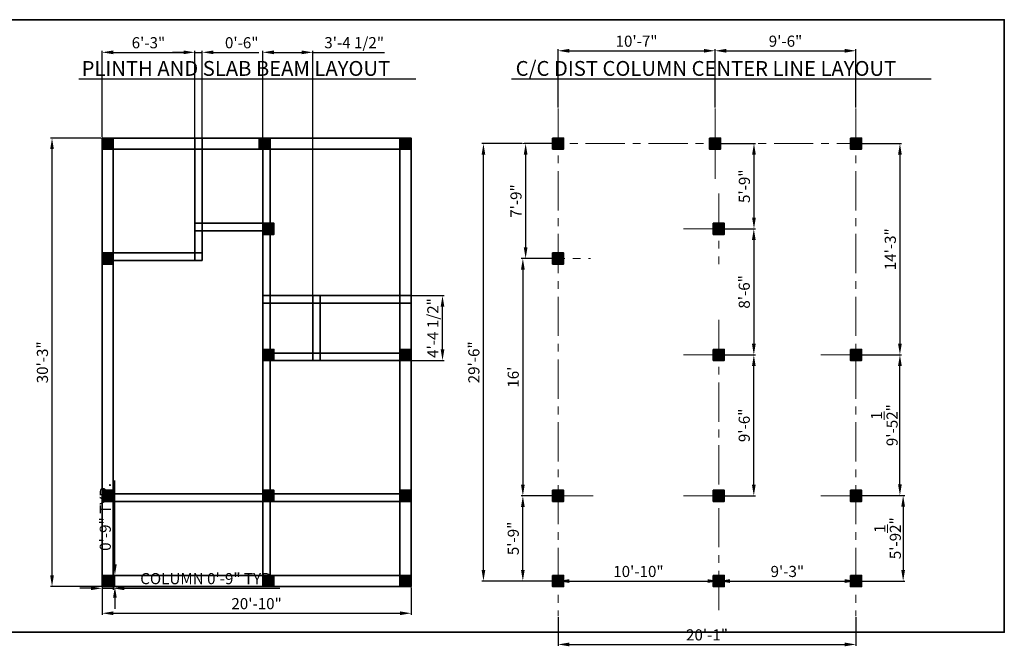
# Model space of a CAD drawing. Units: inches. Extents: x 1838 to 3181, y 1882 to 2430.
# Tile 4 of 4: x 2384 to 3181, y 1882 to 2389. Entities that reach past the tile are written whole.
import ezdxf

# ---------------------------------------------------------------- set-up
doc = ezdxf.new("R2010")
doc.units = ezdxf.units.IN
doc.linetypes.add('CENTER', pattern=[50.8, 31.75, -6.35, 6.35, -6.35])
for name, color, linetype, lineweight in [('A-ANNO-TITL', 6, 'Continuous', 25), ('A-ANNO-TTLB', 7, 'Continuous', 35), ('S-ANNO-DIMS', 2, 'Continuous', 18), ('S-BEAM', 3, 'Continuous', 35), ('S-COLS', 1, 'Continuous', 35), ('S-GRID', 7, 'CENTER', 13)]:
    doc.layers.add(name, color=color, linetype=linetype, lineweight=lineweight)
doc.styles.get("Standard").update_dxf_attribs({"font": 'arial.ttf'})
doc.dimstyles.new('ISO-25', dxfattribs={"dimtxt": 9, "dimasz": 9, "dimexe": 1.25, "dimexo": 0.625, "dimgap": 2, "dimtad": 1, "dimdec": 1, "dimlunit": 4, "dimtxsty": 'Standard', "dimcen": 2.5, "dimadec": 0, "dimazin": 0, "dimtfac": 1, "dimtdec": 1, "dimtmove": 0, "dimatfit": 3, "dimfxl": 1, "dimarcsym": 0})

# ---------------------------------------------------------------- blocks, each defined once
blk = doc.blocks.new('*D5')
at = {"layer": 'Defpoints', "color": 0, "transparency": 16777216}
for p in [(2819.83, 2288.96), (2793.58, 2195.96), (2819.83, 2195.96)]:
    blk.add_point(p, dxfattribs=at)
at = {"layer": 'S-ANNO-DIMS', "color": 0, "lineweight": -2, "transparency": 16777216}
for p, q in [((2819.2, 2288.96), (2792.33, 2288.96)), ((2793.58, 2279.96), (2793.58, 2204.96)), ((2819.2, 2195.96), (2792.33, 2195.96))]:
    blk.add_line(p, q, dxfattribs=at)
at = {"layer": 'S-ANNO-DIMS', "color": 0, "transparency": 16777216}
for points in [[(2792.08, 2279.96), (2795.08, 2279.96), (2793.58, 2288.96)], [(2792.08, 2204.96), (2795.08, 2204.96), (2793.58, 2195.96)]]:
    blk.add_solid(points, dxfattribs=at)
at = {"layer": 'S-ANNO-DIMS', "color": 0, "transparency": 16777216, "insert": (2786.98, 2242.46), "char_height": 9, "attachment_point": 5, "rotation": 90}
blk.add_mtext('7\'-9"', dxfattribs=at)
blk = doc.blocks.new('*D6')
at = {"layer": 'Defpoints', "color": 0, "transparency": 16777216}
for p in [(2819.83, 2195.96), (2791.33, 2003.96), (2819.83, 2003.96)]:
    blk.add_point(p, dxfattribs=at)
at = {"layer": 'S-ANNO-DIMS', "color": 0, "lineweight": -2, "transparency": 16777216}
for p, q in [((2819.2, 2195.96), (2790.08, 2195.96)), ((2791.33, 2186.96), (2791.33, 2012.96)), ((2819.2, 2003.96), (2790.08, 2003.96))]:
    blk.add_line(p, q, dxfattribs=at)
at = {"layer": 'S-ANNO-DIMS', "color": 0, "transparency": 16777216}
for points in [[(2789.83, 2186.96), (2792.83, 2186.96), (2791.33, 2195.96)], [(2789.83, 2012.96), (2792.83, 2012.96), (2791.33, 2003.96)]]:
    blk.add_solid(points, dxfattribs=at)
at = {"layer": 'S-ANNO-DIMS', "color": 0, "transparency": 16777216, "insert": (2784.73, 2099.96), "char_height": 9, "attachment_point": 5, "rotation": 90}
blk.add_mtext("16'", dxfattribs=at)
blk = doc.blocks.new('*D7')
at = {"layer": 'Defpoints', "color": 0, "transparency": 16777216}
for p in [(2791.33, 2003.96), (2804.64, 2003.96), (2819.83, 1934.96)]:
    blk.add_point(p, dxfattribs=at)
at = {"layer": 'S-ANNO-DIMS', "color": 0, "lineweight": -2, "transparency": 16777216}
for p, q in [((2804.02, 2003.96), (2790.08, 2003.96)), ((2791.33, 1943.96), (2791.33, 1994.96)), ((2819.2, 1934.96), (2790.08, 1934.96))]:
    blk.add_line(p, q, dxfattribs=at)
at = {"layer": 'S-ANNO-DIMS', "color": 0, "transparency": 16777216}
for points in [[(2789.83, 1994.96), (2792.83, 1994.96), (2791.33, 2003.96)], [(2789.83, 1943.96), (2792.83, 1943.96), (2791.33, 1934.96)]]:
    blk.add_solid(points, dxfattribs=at)
at = {"layer": 'S-ANNO-DIMS', "color": 0, "transparency": 16777216, "insert": (2784.73, 1969.46), "char_height": 9, "attachment_point": 5, "rotation": 90}
blk.add_mtext('5\'-9"', dxfattribs=at)
blk = doc.blocks.new('*D8')
at = {"layer": 'Defpoints', "color": 0, "transparency": 16777216}
for p in [(2819.83, 1934.96), (2949.83, 1934.96), (2949.83, 1934.96)]:
    blk.add_point(p, dxfattribs=at)
at = {"layer": 'S-ANNO-DIMS', "color": 0, "lineweight": -2, "transparency": 16777216}
for p, q in [((2819.83, 1935.58), (2819.83, 1936.21)), ((2949.83, 1935.58), (2949.83, 1936.21)), ((2828.83, 1934.96), (2940.83, 1934.96))]:
    blk.add_line(p, q, dxfattribs=at)
at = {"layer": 'S-ANNO-DIMS', "color": 0, "transparency": 16777216}
for points in [[(2828.83, 1936.46), (2828.83, 1933.46), (2819.83, 1934.96)], [(2940.83, 1936.46), (2940.83, 1933.46), (2949.83, 1934.96)]]:
    blk.add_solid(points, dxfattribs=at)
at = {"layer": 'S-ANNO-DIMS', "color": 0, "transparency": 16777216, "insert": (2884.83, 1941.55), "char_height": 9, "attachment_point": 5}
blk.add_mtext('10\'-10"', dxfattribs=at)
blk = doc.blocks.new('*D9')
at = {"layer": 'Defpoints', "color": 0, "transparency": 16777216}
for p in [(2949.83, 1935.89), (3060.83, 1934.96), (3060.83, 1934.96)]:
    blk.add_point(p, dxfattribs=at)
at = {"layer": 'S-ANNO-DIMS', "color": 0, "lineweight": -2, "transparency": 16777216}
for p, q in [((2949.83, 1935.27), (2949.83, 1933.71)), ((2958.83, 1934.96), (3051.83, 1934.96)), ((3060.83, 1934.33), (3060.83, 1933.71))]:
    blk.add_line(p, q, dxfattribs=at)
at = {"layer": 'S-ANNO-DIMS', "color": 0, "transparency": 16777216}
for points in [[(2958.83, 1936.46), (2958.83, 1933.46), (2949.83, 1934.96)], [(3051.83, 1936.46), (3051.83, 1933.46), (3060.83, 1934.96)]]:
    blk.add_solid(points, dxfattribs=at)
at = {"layer": 'S-ANNO-DIMS', "color": 0, "transparency": 16777216, "insert": (3005.33, 1941.55), "char_height": 9, "attachment_point": 5}
blk.add_mtext('9\'-3"', dxfattribs=at)
blk = doc.blocks.new('*D10')
at = {"layer": 'Defpoints', "color": 0, "transparency": 16777216}
for p in [(3060.83, 2004.26), (3060.83, 1934.96), (3099.01, 1934.96)]:
    blk.add_point(p, dxfattribs=at)
at = {"layer": 'S-ANNO-DIMS', "color": 0, "lineweight": -2, "transparency": 16777216}
for p, q in [((3061.45, 2004.26), (3100.26, 2004.26)), ((3099.01, 1995.26), (3099.01, 1943.96)), ((3061.45, 1934.96), (3100.26, 1934.96))]:
    blk.add_line(p, q, dxfattribs=at)
at = {"layer": 'S-ANNO-DIMS', "color": 0, "transparency": 16777216}
for points in [[(3097.51, 1995.26), (3100.51, 1995.26), (3099.01, 2004.26)], [(3097.51, 1943.96), (3100.51, 1943.96), (3099.01, 1934.96)]]:
    blk.add_solid(points, dxfattribs=at)
at = {"layer": 'S-ANNO-DIMS', "color": 0, "transparency": 16777216, "insert": (3086.4, 1969.61), "char_height": 9, "attachment_point": 5, "rotation": 90}
blk.add_mtext('5\'-9{\\H1x;\\S1/2;}"', dxfattribs=at)
blk = doc.blocks.new('*D11')
at = {"layer": 'Defpoints', "color": 0, "transparency": 16777216}
for p in [(3066.58, 2117.96), (3096.39, 2117.96), (3086.61, 2004.26)]:
    blk.add_point(p, dxfattribs=at)
at = {"layer": 'S-ANNO-DIMS', "color": 0, "lineweight": -2, "transparency": 16777216}
for p, q in [((3067.2, 2117.96), (3097.64, 2117.96)), ((3096.39, 2013.26), (3096.39, 2108.96)), ((3087.23, 2004.26), (3097.64, 2004.26))]:
    blk.add_line(p, q, dxfattribs=at)
at = {"layer": 'S-ANNO-DIMS', "color": 0, "transparency": 16777216}
for points in [[(3094.89, 2108.96), (3097.89, 2108.96), (3096.39, 2117.96)], [(3094.89, 2013.26), (3097.89, 2013.26), (3096.39, 2004.26)]]:
    blk.add_solid(points, dxfattribs=at)
at = {"layer": 'S-ANNO-DIMS', "color": 0, "transparency": 16777216, "insert": (3083.77, 2061.11), "char_height": 9, "attachment_point": 5, "rotation": 90}
blk.add_mtext('9\'-5{\\H1x;\\S1/2;}"', dxfattribs=at)
blk = doc.blocks.new('*D12')
at = {"layer": 'Defpoints', "color": 0, "transparency": 16777216}
for p in [(3060.83, 2288.96), (3060.83, 2117.96), (3096.39, 2117.96)]:
    blk.add_point(p, dxfattribs=at)
at = {"layer": 'S-ANNO-DIMS', "color": 0, "lineweight": -2, "transparency": 16777216}
for p, q in [((3061.45, 2288.96), (3097.64, 2288.96)), ((3096.39, 2279.96), (3096.39, 2126.96)), ((3061.45, 2117.96), (3097.64, 2117.96))]:
    blk.add_line(p, q, dxfattribs=at)
at = {"layer": 'S-ANNO-DIMS', "color": 0, "transparency": 16777216}
for points in [[(3094.89, 2279.96), (3097.89, 2279.96), (3096.39, 2288.96)], [(3094.89, 2126.96), (3097.89, 2126.96), (3096.39, 2117.96)]]:
    blk.add_solid(points, dxfattribs=at)
at = {"layer": 'S-ANNO-DIMS', "color": 0, "transparency": 16777216, "insert": (3089.79, 2203.46), "char_height": 9, "attachment_point": 5, "rotation": 90}
blk.add_mtext('14\'-3"', dxfattribs=at)
blk = doc.blocks.new('*D13')
at = {"layer": 'Defpoints', "color": 0, "transparency": 16777216}
for p in [(2949.83, 2117.96), (2978.2, 2117.96), (2949.83, 2003.96)]:
    blk.add_point(p, dxfattribs=at)
at = {"layer": 'S-ANNO-DIMS', "color": 0, "lineweight": -2, "transparency": 16777216}
for p, q in [((2950.45, 2117.96), (2979.45, 2117.96)), ((2978.2, 2012.96), (2978.2, 2108.96)), ((2950.45, 2003.96), (2979.45, 2003.96))]:
    blk.add_line(p, q, dxfattribs=at)
at = {"layer": 'S-ANNO-DIMS', "color": 0, "transparency": 16777216}
for points in [[(2976.7, 2108.96), (2979.7, 2108.96), (2978.2, 2117.96)], [(2976.7, 2012.96), (2979.7, 2012.96), (2978.2, 2003.96)]]:
    blk.add_solid(points, dxfattribs=at)
at = {"layer": 'S-ANNO-DIMS', "color": 0, "transparency": 16777216, "insert": (2971.61, 2060.96), "char_height": 9, "attachment_point": 5, "rotation": 90}
blk.add_mtext('9\'-6"', dxfattribs=at)
blk = doc.blocks.new('*D14')
at = {"layer": 'Defpoints', "color": 0, "transparency": 16777216}
for p in [(2949.83, 2219.96), (2949.83, 2117.96), (2978.2, 2117.96)]:
    blk.add_point(p, dxfattribs=at)
at = {"layer": 'S-ANNO-DIMS', "color": 0, "lineweight": -2, "transparency": 16777216}
for p, q in [((2950.45, 2219.96), (2979.45, 2219.96)), ((2978.2, 2210.96), (2978.2, 2126.96)), ((2950.45, 2117.96), (2979.45, 2117.96))]:
    blk.add_line(p, q, dxfattribs=at)
at = {"layer": 'S-ANNO-DIMS', "color": 0, "transparency": 16777216}
for points in [[(2976.7, 2210.96), (2979.7, 2210.96), (2978.2, 2219.96)], [(2976.7, 2126.96), (2979.7, 2126.96), (2978.2, 2117.96)]]:
    blk.add_solid(points, dxfattribs=at)
at = {"layer": 'S-ANNO-DIMS', "color": 0, "transparency": 16777216, "insert": (2971.61, 2168.96), "char_height": 9, "attachment_point": 5, "rotation": 90}
blk.add_mtext('8\'-6"', dxfattribs=at)
blk = doc.blocks.new('*D15')
at = {"layer": 'Defpoints', "color": 0, "transparency": 16777216}
for p in [(2946.83, 2288.96), (2949.83, 2219.96), (2978.33, 2219.96)]:
    blk.add_point(p, dxfattribs=at)
at = {"layer": 'S-ANNO-DIMS', "color": 0, "lineweight": -2, "transparency": 16777216}
for p, q in [((2947.45, 2288.96), (2979.58, 2288.96)), ((2978.33, 2279.96), (2978.33, 2228.96)), ((2950.45, 2219.96), (2979.58, 2219.96))]:
    blk.add_line(p, q, dxfattribs=at)
at = {"layer": 'S-ANNO-DIMS', "color": 0, "transparency": 16777216}
for points in [[(2976.83, 2279.96), (2979.83, 2279.96), (2978.33, 2288.96)], [(2976.83, 2228.96), (2979.83, 2228.96), (2978.33, 2219.96)]]:
    blk.add_solid(points, dxfattribs=at)
at = {"layer": 'S-ANNO-DIMS', "color": 0, "transparency": 16777216, "insert": (2971.73, 2254.46), "char_height": 9, "attachment_point": 5, "rotation": 90}
blk.add_mtext('5\'-9"', dxfattribs=at)
blk = doc.blocks.new('COL-9X9')
h = blk.add_hatch(color=256)
h.dxf.hatch_style = 1
h.paths.add_polyline_path([(9, 9), (0, 9), (0, 0), (9, 0)])
blk.add_lwpolyline([(0, 9), (9, 9), (9, 0), (0, 0)], close=True)
blk = doc.blocks.new('*D21')
at = {"layer": 'Defpoints', "color": 0, "transparency": 16777216}
for p in [(2450.92, 1930.46), (2459.92, 1930.46), (2459.92, 1929.11)]:
    blk.add_point(p, dxfattribs=at)
at = {"layer": 'S-ANNO-DIMS', "color": 0, "lineweight": -2, "transparency": 16777216}
for p, q in [((2441.92, 1929.11), (2432.92, 1929.11)), ((2450.92, 1929.83), (2450.92, 1927.86)), ((2450.92, 1929.11), (2459.92, 1929.11)), ((2459.92, 1929.83), (2459.92, 1927.86)), ((2468.92, 1929.11), (2594.65, 1929.11))]:
    blk.add_line(p, q, dxfattribs=at)
at = {"layer": 'S-ANNO-DIMS', "color": 0, "transparency": 16777216}
for points in [[(2441.92, 1930.61), (2441.92, 1927.61), (2450.92, 1929.11)], [(2468.92, 1930.61), (2468.92, 1927.61), (2459.92, 1929.11)]]:
    blk.add_solid(points, dxfattribs=at)
at = {"layer": 'S-ANNO-DIMS', "color": 0, "transparency": 16777216, "insert": (2536.28, 1935.76), "char_height": 9, "attachment_point": 5}
blk.add_mtext('COLUMN 0\'-9" TYP.', dxfattribs=at)
blk = doc.blocks.new('*D22')
at = {"layer": 'Defpoints', "color": 0, "transparency": 16777216}
for p in [(2459.92, 1939.46), (2461.27, 1939.46), (2459.92, 1930.46)]:
    blk.add_point(p, dxfattribs=at)
at = {"layer": 'S-ANNO-DIMS', "color": 0, "lineweight": -2, "transparency": 16777216}
for p, q in [((2461.27, 1948.46), (2461.27, 2016.32)), ((2460.54, 1939.46), (2462.52, 1939.46)), ((2461.27, 1930.46), (2461.27, 1939.46)), ((2460.54, 1930.46), (2462.52, 1930.46)), ((2461.27, 1921.46), (2461.27, 1912.46))]:
    blk.add_line(p, q, dxfattribs=at)
at = {"layer": 'S-ANNO-DIMS', "color": 0, "transparency": 16777216}
for points in [[(2459.77, 1948.46), (2462.77, 1948.46), (2461.27, 1939.46)], [(2459.77, 1921.46), (2462.77, 1921.46), (2461.27, 1930.46)]]:
    blk.add_solid(points, dxfattribs=at)
at = {"layer": 'S-ANNO-DIMS', "color": 0, "transparency": 16777216, "insert": (2454.67, 1986.89), "char_height": 9, "attachment_point": 5, "rotation": 90}
blk.add_mtext('0\'-9" TYP.', dxfattribs=at)
blk = doc.blocks.new('*D58')
at = {"layer": 'Defpoints', "color": 0, "transparency": 16777216}
for p in [(2450.92, 1930.46), (2700.92, 1930.46), (2700.92, 1908.91)]:
    blk.add_point(p, dxfattribs=at)
at = {"layer": 'S-ANNO-DIMS', "color": 0, "lineweight": -2, "transparency": 16777216}
for p, q in [((2450.92, 1929.83), (2450.92, 1907.66)), ((2700.92, 1929.83), (2700.92, 1907.66)), ((2459.92, 1908.91), (2691.92, 1908.91))]:
    blk.add_line(p, q, dxfattribs=at)
at = {"layer": 'S-ANNO-DIMS', "color": 0, "transparency": 16777216}
for points in [[(2459.92, 1910.41), (2459.92, 1907.41), (2450.92, 1908.91)], [(2691.92, 1910.41), (2691.92, 1907.41), (2700.92, 1908.91)]]:
    blk.add_solid(points, dxfattribs=at)
at = {"layer": 'S-ANNO-DIMS', "color": 0, "transparency": 16777216, "insert": (2575.92, 1915.5), "char_height": 9, "attachment_point": 5}
blk.add_mtext('20\'-10"', dxfattribs=at)
blk = doc.blocks.new('*D59')
at = {"layer": 'Defpoints', "color": 0, "transparency": 16777216}
for p in [(2410.42, 2293.46), (2450.92, 2293.46), (2450.92, 1930.46)]:
    blk.add_point(p, dxfattribs=at)
at = {"layer": 'S-ANNO-DIMS', "color": 0, "lineweight": -2, "transparency": 16777216}
for p, q in [((2450.29, 2293.46), (2409.17, 2293.46)), ((2410.42, 1939.46), (2410.42, 2284.46)), ((2450.29, 1930.46), (2409.17, 1930.46))]:
    blk.add_line(p, q, dxfattribs=at)
at = {"layer": 'S-ANNO-DIMS', "color": 0, "transparency": 16777216}
for points in [[(2408.92, 2284.46), (2411.92, 2284.46), (2410.42, 2293.46)], [(2408.92, 1939.46), (2411.92, 1939.46), (2410.42, 1930.46)]]:
    blk.add_solid(points, dxfattribs=at)
at = {"layer": 'S-ANNO-DIMS', "color": 0, "transparency": 16777216, "insert": (2403.82, 2111.96), "char_height": 9, "attachment_point": 5, "rotation": 90}
blk.add_mtext('30\'-3"', dxfattribs=at)
blk = doc.blocks.new('*D60')
at = {"layer": 'Defpoints', "color": 0, "transparency": 16777216}
for p in [(2525.92, 2362.81), (2450.92, 2293.46), (2525.92, 2293.46)]:
    blk.add_point(p, dxfattribs=at)
at = {"layer": 'S-ANNO-DIMS', "color": 0, "lineweight": -2, "transparency": 16777216}
for p, q in [((2450.92, 2294.08), (2450.92, 2364.06)), ((2459.92, 2362.81), (2516.92, 2362.81)), ((2525.92, 2294.08), (2525.92, 2364.06))]:
    blk.add_line(p, q, dxfattribs=at)
at = {"layer": 'S-ANNO-DIMS', "color": 0, "transparency": 16777216}
for points in [[(2459.92, 2364.31), (2459.92, 2361.31), (2450.92, 2362.81)], [(2516.92, 2364.31), (2516.92, 2361.31), (2525.92, 2362.81)]]:
    blk.add_solid(points, dxfattribs=at)
at = {"layer": 'S-ANNO-DIMS', "color": 0, "transparency": 16777216, "insert": (2488.42, 2369.41), "char_height": 9, "attachment_point": 5}
blk.add_mtext('6\'-3"', dxfattribs=at)
blk = doc.blocks.new('*D61')
at = {"layer": 'Defpoints', "color": 0, "transparency": 16777216}
for p in [(2621.42, 2362.81), (2580.92, 2165.96), (2621.42, 2165.96)]:
    blk.add_point(p, dxfattribs=at)
at = {"layer": 'S-ANNO-DIMS', "color": 0, "lineweight": -2, "transparency": 16777216}
for p, q in [((2580.92, 2166.58), (2580.92, 2364.06)), ((2589.92, 2362.81), (2612.42, 2362.81)), ((2621.42, 2166.58), (2621.42, 2364.06)), ((2621.42, 2362.81), (2679.31, 2362.81))]:
    blk.add_line(p, q, dxfattribs=at)
at = {"layer": 'S-ANNO-DIMS', "color": 0, "transparency": 16777216}
for points in [[(2589.92, 2364.31), (2589.92, 2361.31), (2580.92, 2362.81)], [(2612.42, 2364.31), (2612.42, 2361.31), (2621.42, 2362.81)]]:
    blk.add_solid(points, dxfattribs=at)
at = {"layer": 'S-ANNO-DIMS', "color": 0, "transparency": 16777216, "insert": (2654.86, 2369.47), "char_height": 9, "attachment_point": 5}
blk.add_mtext('3\'-4 1/2"', dxfattribs=at)
blk = doc.blocks.new('*D62')
at = {"layer": 'Defpoints', "color": 0, "transparency": 16777216}
for p in [(2700.92, 2165.96), (2726.33, 2165.96), (2700.92, 2113.46)]:
    blk.add_point(p, dxfattribs=at)
at = {"layer": 'S-ANNO-DIMS', "color": 0, "lineweight": -2, "transparency": 16777216}
for p, q in [((2701.54, 2165.96), (2727.58, 2165.96)), ((2726.33, 2122.46), (2726.33, 2156.96)), ((2701.54, 2113.46), (2727.58, 2113.46))]:
    blk.add_line(p, q, dxfattribs=at)
at = {"layer": 'S-ANNO-DIMS', "color": 0, "transparency": 16777216}
for points in [[(2724.83, 2156.96), (2727.83, 2156.96), (2726.33, 2165.96)], [(2724.83, 2122.46), (2727.83, 2122.46), (2726.33, 2113.46)]]:
    blk.add_solid(points, dxfattribs=at)
at = {"layer": 'S-ANNO-DIMS', "color": 0, "transparency": 16777216, "insert": (2719.67, 2139.71), "char_height": 9, "attachment_point": 5, "rotation": 90}
blk.add_mtext('4\'-4 1/2"', dxfattribs=at)
blk = doc.blocks.new('*D63')
at = {"layer": 'Defpoints', "color": 0, "transparency": 16777216}
for p in [(2531.92, 2362.81), (2525.92, 2293.46), (2531.92, 2293.46)]:
    blk.add_point(p, dxfattribs=at)
at = {"layer": 'S-ANNO-DIMS', "color": 0, "lineweight": -2, "transparency": 16777216}
for p, q in [((2516.92, 2362.81), (2507.92, 2362.81)), ((2525.92, 2294.08), (2525.92, 2364.06)), ((2525.92, 2362.81), (2531.92, 2362.81)), ((2531.92, 2294.08), (2531.92, 2364.06)), ((2540.92, 2362.81), (2577.84, 2362.81))]:
    blk.add_line(p, q, dxfattribs=at)
at = {"layer": 'S-ANNO-DIMS', "color": 0, "transparency": 16777216}
for points in [[(2516.92, 2364.31), (2516.92, 2361.31), (2525.92, 2362.81)], [(2540.92, 2364.31), (2540.92, 2361.31), (2531.92, 2362.81)]]:
    blk.add_solid(points, dxfattribs=at)
at = {"layer": 'S-ANNO-DIMS', "color": 0, "transparency": 16777216, "insert": (2563.88, 2369.41), "char_height": 9, "attachment_point": 5}
blk.add_mtext('0\'-6"', dxfattribs=at)
blk = doc.blocks.new('*D64')
at = {"layer": 'Defpoints', "color": 0, "transparency": 16777216}
for p in [(2819.83, 1906.46), (3060.83, 1906.46), (3060.83, 1883.66)]:
    blk.add_point(p, dxfattribs=at)
at = {"layer": 'S-ANNO-DIMS', "color": 0, "lineweight": -2, "transparency": 16777216}
for p, q in [((2819.83, 1905.83), (2819.83, 1882.41)), ((3060.83, 1905.83), (3060.83, 1882.41)), ((2828.83, 1883.66), (3051.83, 1883.66))]:
    blk.add_line(p, q, dxfattribs=at)
at = {"layer": 'S-ANNO-DIMS', "color": 0, "transparency": 16777216}
for points in [[(2828.83, 1885.16), (2828.83, 1882.16), (2819.83, 1883.66)], [(3051.83, 1885.16), (3051.83, 1882.16), (3060.83, 1883.66)]]:
    blk.add_solid(points, dxfattribs=at)
at = {"layer": 'S-ANNO-DIMS', "color": 0, "transparency": 16777216, "insert": (2940.33, 1890.25), "char_height": 9, "attachment_point": 5}
blk.add_mtext('20\'-1"', dxfattribs=at)
blk = doc.blocks.new('*D65')
at = {"layer": 'Defpoints', "color": 0, "transparency": 16777216}
for p in [(2759.46, 2288.96), (2791.33, 2288.96), (2800.83, 1934.96)]:
    blk.add_point(p, dxfattribs=at)
at = {"layer": 'S-ANNO-DIMS', "color": 0, "lineweight": -2, "transparency": 16777216}
for p, q in [((2790.7, 2288.96), (2758.21, 2288.96)), ((2759.46, 1943.96), (2759.46, 2279.96)), ((2800.2, 1934.96), (2758.21, 1934.96))]:
    blk.add_line(p, q, dxfattribs=at)
at = {"layer": 'S-ANNO-DIMS', "color": 0, "transparency": 16777216}
for points in [[(2757.96, 2279.96), (2760.96, 2279.96), (2759.46, 2288.96)], [(2757.96, 1943.96), (2760.96, 1943.96), (2759.46, 1934.96)]]:
    blk.add_solid(points, dxfattribs=at)
at = {"layer": 'S-ANNO-DIMS', "color": 0, "transparency": 16777216, "insert": (2752.87, 2111.96), "char_height": 9, "attachment_point": 5, "rotation": 90}
blk.add_mtext('29\'-6"', dxfattribs=at)
blk = doc.blocks.new('*D66')
at = {"layer": 'Defpoints', "color": 0, "transparency": 16777216}
for p in [(2946.83, 2364.06), (2819.83, 2317.46), (2946.83, 2317.46)]:
    blk.add_point(p, dxfattribs=at)
at = {"layer": 'S-ANNO-DIMS', "color": 0, "lineweight": -2, "transparency": 16777216}
for p, q in [((2819.83, 2318.08), (2819.83, 2365.31)), ((2828.83, 2364.06), (2937.83, 2364.06)), ((2946.83, 2318.08), (2946.83, 2365.31))]:
    blk.add_line(p, q, dxfattribs=at)
at = {"layer": 'S-ANNO-DIMS', "color": 0, "transparency": 16777216}
for points in [[(2828.83, 2365.56), (2828.83, 2362.56), (2819.83, 2364.06)], [(2937.83, 2365.56), (2937.83, 2362.56), (2946.83, 2364.06)]]:
    blk.add_solid(points, dxfattribs=at)
at = {"layer": 'S-ANNO-DIMS', "color": 0, "transparency": 16777216, "insert": (2883.33, 2370.66), "char_height": 9, "attachment_point": 5}
blk.add_mtext('10\'-7"', dxfattribs=at)
blk = doc.blocks.new('*D67')
at = {"layer": 'Defpoints', "color": 0, "transparency": 16777216}
for p in [(3060.83, 2364.06), (2946.83, 2317.46), (3060.83, 2317.46)]:
    blk.add_point(p, dxfattribs=at)
at = {"layer": 'S-ANNO-DIMS', "color": 0, "lineweight": -2, "transparency": 16777216}
for p, q in [((2946.83, 2318.08), (2946.83, 2365.31)), ((2955.83, 2364.06), (3051.83, 2364.06)), ((3060.83, 2318.08), (3060.83, 2365.31))]:
    blk.add_line(p, q, dxfattribs=at)
at = {"layer": 'S-ANNO-DIMS', "color": 0, "transparency": 16777216}
for points in [[(2955.83, 2365.56), (2955.83, 2362.56), (2946.83, 2364.06)], [(3051.83, 2365.56), (3051.83, 2362.56), (3060.83, 2364.06)]]:
    blk.add_solid(points, dxfattribs=at)
at = {"layer": 'S-ANNO-DIMS', "color": 0, "transparency": 16777216, "insert": (3003.83, 2370.66), "char_height": 9, "attachment_point": 5}
blk.add_mtext('9\'-6"', dxfattribs=at)

msp = doc.modelspace()

# ---------------------------------------------------------------- linework, layer by layer
at = {"layer": 'A-ANNO-TITL'}
for p, q in [((2431.97, 2341.26), (2704.78, 2341.26)), ((2782.26, 2341.26), (3121.81, 2341.26))]:
    msp.add_line(p, q, dxfattribs=at)
at = {"layer": 'A-ANNO-TTLB'}
msp.add_lwpolyline([(1905.37, 2389.23), (3180.85, 2389.23), (3180.85, 1893.51), (1905.37, 1893.51)], close=True, dxfattribs=at)
at = {"layer": 'S-BEAM'}
for p, q in [((2450.92, 2293.46), (2700.92, 2293.46)), ((2450.92, 2293.46), (2450.92, 1930.46)), ((2459.92, 2293.46), (2459.92, 2200.46)), ((2459.92, 2293.46), (2459.92, 1930.46)), ((2525.92, 2293.46), (2525.92, 2194.46)), ((2531.92, 2293.46), (2531.92, 2194.46)), ((2580.92, 2293.46), (2580.92, 1930.46)), ((2586.92, 2293.46), (2586.92, 1930.46)), ((2691.92, 2293.46), (2691.92, 1930.46)), ((2700.92, 2293.46), (2700.92, 1930.46)), ((2450.92, 2284.46), (2700.92, 2284.46)), ((2525.92, 2224.46), (2586.92, 2224.46)), ((2525.92, 2218.46), (2586.92, 2218.46)), ((2450.92, 2200.46), (2531.92, 2200.46)), ((2450.92, 2194.46), (2531.92, 2194.46)), ((2580.92, 2165.96), (2700.92, 2165.96)), ((2580.92, 2159.96), (2700.92, 2159.96)), ((2621.42, 2165.96), (2621.42, 2113.46)), ((2627.42, 2165.96), (2627.42, 2113.46)), ((2580.92, 2119.46), (2700.92, 2119.46)), ((2580.92, 2113.46), (2700.92, 2113.46)), ((2450.92, 2005.46), (2700.92, 2005.46)), ((2450.92, 1999.46), (2700.92, 1999.46)), ((2450.92, 1939.46), (2700.92, 1939.46)), ((2450.92, 1930.46), (2700.92, 1930.46))]:
    msp.add_line(p, q, dxfattribs=at)
at = {"layer": 'S-COLS'}
for p, q in [((2942.33, 2293.46), (2942.33, 2284.46)), ((2951.33, 2293.46), (2951.33, 2284.46))]:
    msp.add_line(p, q, dxfattribs=at)
at = {"layer": 'S-GRID'}
for p, q in [((2819.83, 2317.46), (2819.83, 1906.46)), ((2946.83, 2317.46), (2946.83, 2284.46)), ((3060.83, 2317.46), (3060.83, 1906.46)), ((2791.33, 2288.96), (3089.33, 2288.96)), ((2946.83, 2284.46), (2946.83, 2260.46)), ((2949.83, 2248.46), (2949.83, 2191.46)), ((2921.33, 2219.96), (2945.33, 2219.96)), ((2954.33, 2219.96), (2978.33, 2219.96)), ((2793.58, 2195.96), (2846.08, 2195.96)), ((2949.83, 2146.46), (2949.83, 1906.46)), ((2921.33, 2117.96), (2945.33, 2117.96)), ((2945.33, 2117.96), (2978.33, 2117.96)), ((3032.33, 2117.96), (3056.33, 2117.96)), ((3056.33, 2117.96), (3089.33, 2117.96)), ((2791.33, 2003.96), (2815.33, 2003.96)), ((2824.33, 2003.96), (2848.33, 2003.96)), ((2921.33, 2003.96), (2945.33, 2003.96)), ((2945.33, 2003.96), (2978.33, 2003.96)), ((3032.33, 2003.96), (3056.33, 2003.96)), ((3065.33, 2003.96), (3089.33, 2003.96)), ((2800.83, 1934.96), (3098.83, 1934.96))]:
    msp.add_line(p, q, dxfattribs=at)

# ---------------------------------------------------------------- block references
at = {"layer": 'S-COLS'}
for p in [(2450.92, 2284.46), (2577.92, 2284.46), (2691.92, 2284.46), (2815.33, 2284.46), (2942.33, 2284.46), (3056.33, 2284.46), (2580.92, 2215.46), (2945.33, 2215.46), (2450.92, 2191.46), (2815.33, 2191.46), (2580.92, 2113.46), (2691.92, 2113.46), (2945.33, 2113.46), (3056.33, 2113.46), (2450.92, 1999.46), (2580.92, 1999.46), (2691.92, 1999.46), (2815.33, 1999.46), (2945.33, 1999.46), (3056.33, 1999.46), (2450.92, 1930.46), (2580.92, 1930.46), (2691.92, 1930.46), (2815.33, 1930.46), (2945.33, 1930.46), (3056.33, 1930.46)]:
    msp.add_blockref('COL-9X9', p, dxfattribs=at)

# ---------------------------------------------------------------- texts
at = {"layer": 'A-ANNO-TITL'}
for s, p in [('PLINTH AND SLAB BEAM LAYOUT', (2434.37, 2343.79)), ('C/C DIST COLUMN CENTER LINE LAYOUT', (2785.5, 2343.79))]:
    msp.add_text(s, height=12, dxfattribs=at).set_placement(p)

# ---------------------------------------------------------------- dimensions: what is measured, and where the dimension line sits
at = {"layer": 'S-ANNO-DIMS'}
for base, p1, p2, override, picture, middle in [((2621.42, 2362.81), (2580.92, 2165.96), (2621.42, 2165.96), {"dimdec": 1, "dimlfac": 1, "dimrnd": 0, "dimzin": 1, "dimdsep": 46, "dimlunit": 4, "dimfrac": 2}, '*D61', (2654.86, 2369.47)), ((2525.92, 2362.81), (2450.92, 2293.46), (2525.92, 2293.46), {"dimdec": 1, "dimlfac": 1, "dimrnd": 0, "dimzin": 1, "dimdsep": 46, "dimlunit": 4, "dimfrac": 2}, '*D60', (2488.42, 2369.41)), ((2531.92, 2362.81), (2525.92, 2293.46), (2531.92, 2293.46), {"dimdec": 1, "dimlfac": 1, "dimrnd": 0, "dimzin": 1, "dimdsep": 46, "dimlunit": 4, "dimfrac": 2}, '*D63', (2563.88, 2369.41)), ((2946.83, 2364.06), (2819.83, 2317.46), (2946.83, 2317.46), {"dimdec": 1, "dimlfac": 1, "dimrnd": 0, "dimzin": 1, "dimdsep": 46, "dimlunit": 4, "dimfrac": 2}, '*D66', (2883.33, 2370.66)), ((3060.83, 2364.06), (2946.83, 2317.46), (3060.83, 2317.46), {"dimdec": 1, "dimlfac": 1, "dimrnd": 0, "dimzin": 1, "dimdsep": 46, "dimlunit": 4, "dimfrac": 2}, '*D67', (3003.83, 2370.66)), ((2949.83, 1934.96), (2819.83, 1934.96), (2949.83, 1934.96), {"dimclrd": 0, "dimclre": 0, "dimclrt": 0}, '*D8', (2884.83, 1941.55)), ((3060.83, 1934.96), (2949.83, 1935.89), (3060.83, 1934.96), {"dimclrd": 0, "dimclre": 0, "dimclrt": 0}, '*D9', (3005.33, 1941.55)), ((2700.92, 1908.91), (2450.92, 1930.46), (2700.92, 1930.46), {"dimdec": 1, "dimlfac": 1, "dimrnd": 0, "dimzin": 1, "dimdsep": 46, "dimlunit": 4, "dimfrac": 2}, '*D58', (2575.92, 1915.5)), ((3060.83, 1883.66), (2819.83, 1906.46), (3060.83, 1906.46), {"dimdec": 1, "dimlfac": 1, "dimrnd": 0, "dimzin": 1, "dimdsep": 46, "dimlunit": 4, "dimfrac": 2}, '*D64', (2940.33, 1890.25))]:
    dim = msp.add_linear_dim(base=base, p1=p1, p2=p2, dimstyle='ISO-25', override=override, dxfattribs=at)
    dim.commit()
    dim.dimension.update_dxf_attribs({"geometry": picture, "text_midpoint": middle})
for base, p1, p2, override, picture, middle in [((2410.42, 2293.46), (2450.92, 1930.46), (2450.92, 2293.46), {"dimdec": 1, "dimlfac": 1, "dimrnd": 0, "dimzin": 1, "dimdsep": 46, "dimlunit": 4, "dimfrac": 2}, '*D59', (2403.82, 2111.96)), ((2759.46, 2288.96), (2800.83, 1934.96), (2791.33, 2288.96), {"dimdec": 1, "dimlfac": 1, "dimrnd": 0, "dimzin": 1, "dimdsep": 46, "dimlunit": 4, "dimfrac": 2}, '*D65', (2752.87, 2111.96)), ((2793.58, 2195.96), (2819.83, 2288.96), (2819.83, 2195.96), {"dimclrd": 0, "dimclre": 0, "dimclrt": 0}, '*D5', (2786.98, 2242.46)), ((2978.33, 2219.96), (2946.83, 2288.96), (2949.83, 2219.96), {"dimclrd": 0, "dimclre": 0, "dimclrt": 0}, '*D15', (2971.73, 2254.46)), ((3096.39, 2117.96), (3060.83, 2288.96), (3060.83, 2117.96), {"dimclrd": 0, "dimclre": 0, "dimclrt": 0}, '*D12', (3089.79, 2203.46)), ((2978.2, 2117.96), (2949.83, 2219.96), (2949.83, 2117.96), {"dimclrd": 0, "dimclre": 0, "dimclrt": 0}, '*D14', (2971.61, 2168.96)), ((2791.33, 2003.96), (2819.83, 2195.96), (2819.83, 2003.96), {"dimclrd": 0, "dimclre": 0, "dimclrt": 0}, '*D6', (2784.73, 2099.96)), ((2726.33, 2165.96), (2700.92, 2113.46), (2700.92, 2165.96), {"dimdec": 1, "dimlfac": 1, "dimrnd": 0, "dimzin": 1, "dimdsep": 46, "dimlunit": 4, "dimfrac": 2}, '*D62', (2719.67, 2139.71)), ((2978.2, 2117.96), (2949.83, 2003.96), (2949.83, 2117.96), {"dimclrd": 0, "dimclre": 0, "dimclrt": 0}, '*D13', (2971.61, 2060.96)), ((3096.39, 2117.96), (3086.61, 2004.26), (3066.58, 2117.96), {"dimclrd": 0, "dimclre": 0, "dimclrt": 0}, '*D11', (3083.77, 2061.11)), ((2791.33, 2003.96), (2819.83, 1934.96), (2804.64, 2003.96), {"dimclrd": 0, "dimclre": 0, "dimclrt": 0}, '*D7', (2784.73, 1969.46)), ((3099.01, 1934.96), (3060.83, 2004.26), (3060.83, 1934.96), {"dimclrd": 0, "dimclre": 0, "dimclrt": 0}, '*D10', (3086.4, 1969.61))]:
    dim = msp.add_linear_dim(base=base, p1=p1, p2=p2, angle=90, dimstyle='ISO-25', override=override, dxfattribs=at)
    dim.commit()
    dim.dimension.update_dxf_attribs({"geometry": picture, "text_midpoint": middle})
dim = msp.add_linear_dim(base=(2461.27, 1939.46), p1=(2459.92, 1930.46), p2=(2459.92, 1939.46), angle=90, text='<> TYP.', dimstyle='ISO-25', override={"dimdec": 1, "dimlfac": 1, "dimrnd": 0, "dimzin": 1, "dimdsep": 46, "dimlunit": 4, "dimfrac": 2}, dxfattribs=at)
dim.commit()
dim.dimension.update_dxf_attribs({"geometry": '*D22', "text_midpoint": (2454.67, 1986.89)})
dim = msp.add_linear_dim(base=(2459.92, 1929.11), p1=(2450.92, 1930.46), p2=(2459.92, 1930.46), text='COLUMN <> TYP.', dimstyle='ISO-25', override={"dimdec": 1, "dimlfac": 1, "dimrnd": 0, "dimzin": 1, "dimdsep": 46, "dimlunit": 4, "dimfrac": 2}, dxfattribs=at)
dim.commit()
dim.dimension.update_dxf_attribs({"geometry": '*D21', "text_midpoint": (2536.28, 1935.76)})

doc.saveas('drawing.dxf')
